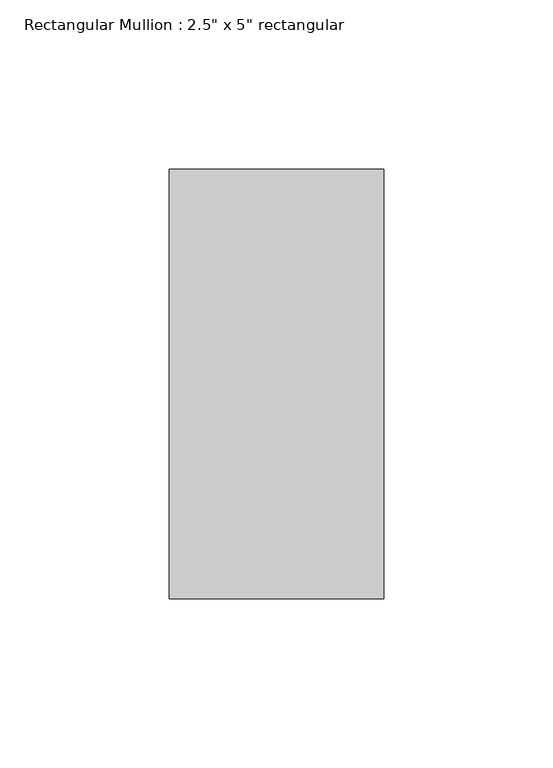
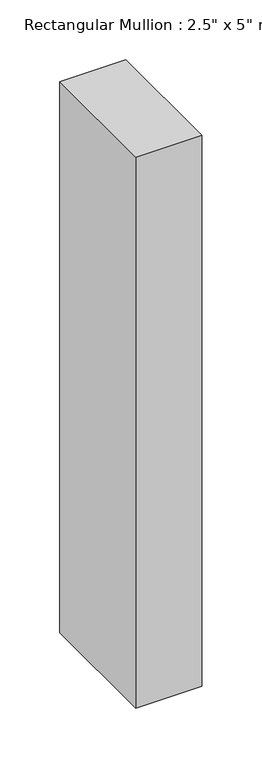
"""IFC4 building model written with IfcOpenShell, lengths in millimetres: member geometry."""

from ifc_helpers import new_model, si_unit, frame, origin, place, context, project, spatial, polyline, outline, extrude, source, transform, mapped, element, save


def member_8e397d51(model_context):
    return source(origin(), model_context, "Body", "SweptSolid", [
        extrude(outline(polyline([(0.0, 63.5), (0.0, -63.5), (-63.5, -63.5), (-63.5, 63.5), (0.0, 63.5)])), frame((0.0, 0.0, -561.975), z_axis=(0.0, 0.0, 1.0), x_axis=(1.0, 0.0, 0.0)), (0.0, 0.0, 1.0), 561.975),
    ])


if __name__ == "__main__":
    model = new_model("IFC4")
    model_context = context("Model", 3, world=origin())
    ifc_project = project(units=[si_unit("LENGTHUNIT", "METRE", prefix="MILLI")], contexts=[model_context])
    site = spatial("IfcSite", under=ifc_project)
    building = spatial("IfcBuilding", under=site)
    placement = place(None, origin())
    member_shape = member_8e397d51(model_context)
    element("IfcMember", 1, ObjectType="Rectangular Mullion : 2.5\" x 5\" rectangular", at=placement, inside=building, context=model_context, shape_type="MappedRepresentation", body=[
        mapped(member_shape, transform((0.0, 0.0, 0.0), x_axis=(1.0, 0.0, 0.0), y_axis=(0.0, 1.0, 0.0), z_axis=(0.0, 0.0, 1.0))),
    ])
    save(model, "model.ifc")

# Revit data of these elements
# Type "Rectangular Mullion : 2.5\" x 5\" rectangular"
#   built-in parameter 1007304 = 0.416667 (stored number, unit not read)
#   built-in parameter 1007301 = 0.104167 (stored number, unit not read)
#   built-in parameter 1007300 = 0.104167 (stored number, unit not read)
# Element 1 (IfcMember, "Rectangular Mullion : 2.5\" x 5\" rectangular")
#   Materials on its faces: "Aluminum"
# Materials
#   "Aluminum": class "Metal", colour RGB 247 247 247, transparency 0, Description = "Aluminum 6061", Cost = 0
